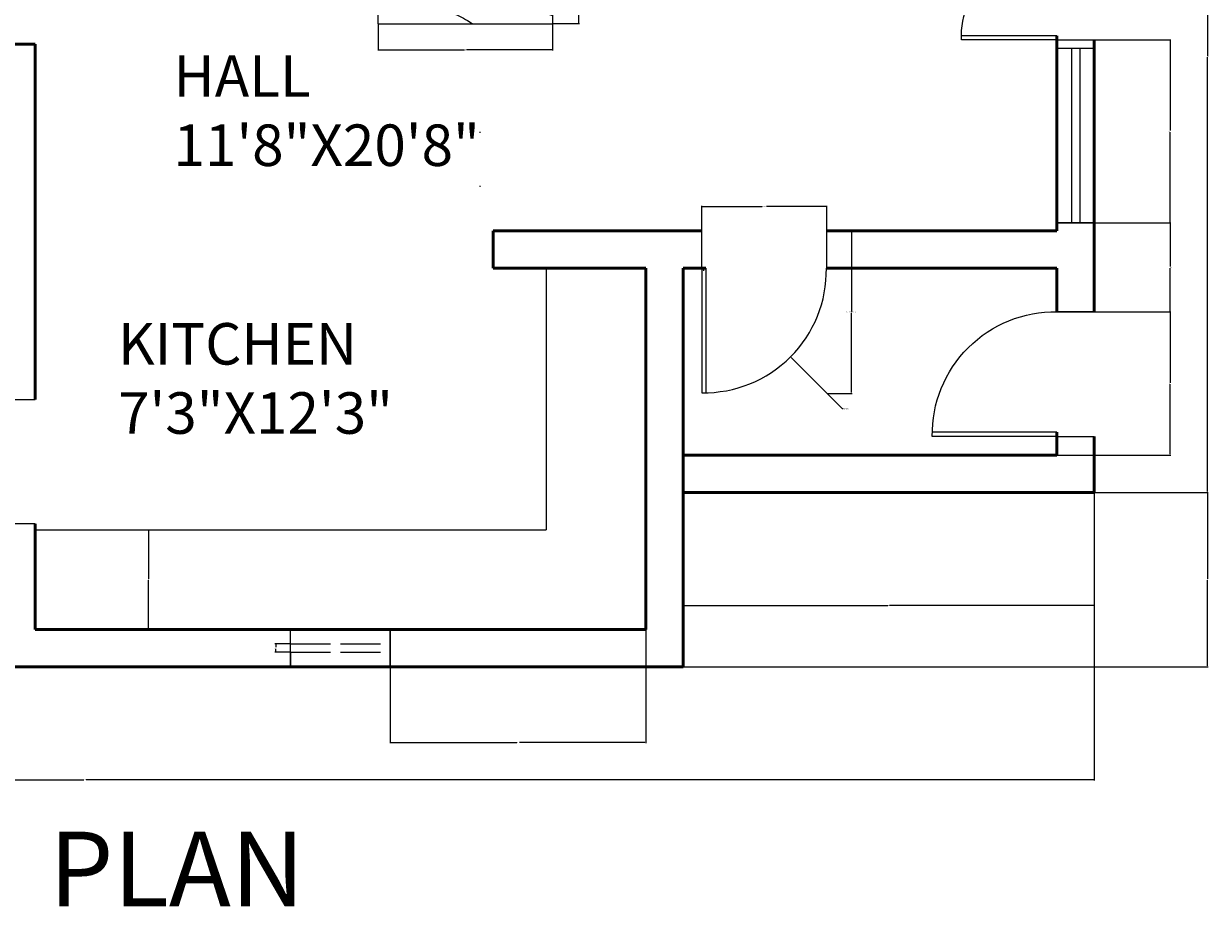
# Model space of a CAD drawing. Units: inches. Extents: x 178 to 719, y 262 to 748.
# Tile 2 of 3: x 434 to 719, y 262 to 475. Entities that reach past the tile are written whole.
import ezdxf

# ---------------------------------------------------------------- set-up
doc = ezdxf.new("R2010")
doc.units = ezdxf.units.IN
doc.linetypes.add('ACAD_ISO02W100', pattern=[15, 12, -3])
for name, color, linetype, lineweight in [('A-ANNO-DIMS', 2, 'Continuous', 18), ('A-ANNO-TEXT', 7, 'Continuous', 35), ('A-AREA-IDEN', 7, 'Continuous', 25), ('A-DOOR', 3, 'Continuous', 25), ('A-FLOR-CASE', 32, 'Continuous', 25), ('A-FURN', 8, 'Continuous', 18), ('A-GLAZ', 4, 'Continuous', 18), ('A-GLAZ-OVHD', 4, 'ACAD_ISO02W100', 18), ('A-WALL', 7, 'Continuous', 50)]:
    doc.layers.add(name, color=color, linetype=linetype, lineweight=lineweight)
doc.styles.get("Standard").update_dxf_attribs({"font": 'arial.ttf'})
doc.dimstyles.get("Standard").update_dxf_attribs({"dimtxt": 0.18, "dimasz": 0.18, "dimexe": 0.18, "dimexo": 0.0625, "dimgap": 0.09, "dimtad": 0, "dimtih": 1, "dimtoh": 1, "dimdec": 4, "dimzin": 0, "dimdsep": 46, "dimtxsty": 'Standard', "dimcen": 0.09, "dimadec": 0, "dimazin": 0, "dimtfac": 1, "dimtdec": 4, "dimtofl": 0, "dimtmove": 0, "dimatfit": 3, "dimfxl": 1, "dimtolj": 1, "dimtzin": 0, "dimarcsym": 0})

# ---------------------------------------------------------------- blocks, each defined once
blk = doc.blocks.new('Table - Square Woodgrain 42 x 42 in.')
blk.add_line((0, -42), (42, -42))
for points in [[(0, -4), (1.704, -4.2172), (3.2358, -4.4188), (4.615, -4.604), (5.8615, -4.7721), (6.9951, -4.9224), (8.0357, -5.0541), (9.0031, -5.1667), (9.9171, -5.2594), (10.7951, -5.3316), (11.6445, -5.3836), (12.4702, -5.4157), (13.277, -5.4283), (14.0698, -5.4217), (14.8535, -5.3964), (15.6331, -5.3526), (16.4133, -5.2908), (17.1986, -5.2103), (17.9913, -5.1062), (18.793, -4.9727), (19.6056, -4.8038), (20.4307, -4.5937), (21.2701, -4.3365), (22.1256, -4.0262), (22.9989, -3.6571), (23.888, -3.2272), (24.7756, -2.7516), (25.6408, -2.2491), (26.4624, -1.7387), (27.2195, -1.2395), (27.891, -0.7703), (28.456, -0.3501), (28.8934, 0.002)], [(0, -42), (0, 0), (42, 0), (42, -42)], [(0, -8), (1.8203, -8.1001), (3.6741, -8.2149), (5.5411, -8.3408), (7.4011, -8.4741), (9.2339, -8.6112), (11.0193, -8.7484), (12.7371, -8.8821), (14.3671, -9.0086), (15.8954, -9.1246), (17.3337, -9.2278), (18.6997, -9.3159), (20.0116, -9.387), (21.2871, -9.4389), (22.5442, -9.4696), (23.8008, -9.477), (25.0749, -9.459), (26.3791, -9.4137), (27.7049, -9.3403), (29.0383, -9.2382), (30.3655, -9.1068), (31.6728, -8.9455), (32.9461, -8.7535), (34.1717, -8.5304), (35.3358, -8.2756), (36.4268, -7.9863), (37.443, -7.6521), (38.3849, -7.2603), (39.253, -6.7986), (40.048, -6.2542), (40.7705, -5.6147), (41.421, -4.8674), (42, -4)], [(42, -12), (39.1784, -12.8621), (36.4519, -13.5654), (33.8246, -14.1294), (31.3004, -14.5731), (28.8832, -14.9161), (26.577, -15.1775), (24.3858, -15.3768), (22.3136, -15.5332), (20.3622, -15.6632), (18.5254, -15.7718), (16.7947, -15.8612), (15.1618, -15.9338), (13.6183, -15.9916), (12.1558, -16.0369), (10.7659, -16.0718), (9.4403, -16.0987), (8.1703, -16.1191), (6.9461, -16.1325), (5.7577, -16.1377), (4.595, -16.1335), (3.4479, -16.1188), (2.3064, -16.0924), (1.1604, -16.0532), (0, -16)], [(42, -16), (37.6529, -16.7365), (33.8802, -17.329), (30.6179, -17.7961), (27.8015, -18.1561), (25.3668, -18.4275), (23.2497, -18.6288), (21.3859, -18.7785), (19.7111, -18.8949), (18.1693, -18.9939), (16.7375, -19.0795), (15.401, -19.1534), (14.1449, -19.217), (12.9544, -19.2717), (11.8148, -19.3191), (10.7113, -19.3606), (9.6291, -19.3976), (8.5534, -19.4323), (7.47, -19.4689), (6.3643, -19.5122), (5.222, -19.5672), (4.0288, -19.6386), (2.7703, -19.7313), (1.4321, -19.8501), (0, -20)], [(0, -24), (3.9243, -23.6805), (7.4766, -23.4138), (10.6891, -23.1954), (13.5943, -23.0205), (16.2247, -22.8847), (18.6125, -22.7832), (20.7903, -22.7116), (22.7903, -22.6651), (24.6563, -22.642), (26.4764, -22.6507), (28.35, -22.7024), (30.3766, -22.8084), (32.6555, -22.98), (35.2861, -23.2283), (38.3678, -23.5645), (42, -24)], [(42, -32), (37.392, -31.017), (33.4585, -30.2231), (30.1291, -29.5949), (27.3334, -29.109), (25.0009, -28.742), (23.0612, -28.4707), (21.4439, -28.2716), (20.0786, -28.1215), (18.8998, -28.0002), (17.8609, -27.9014), (16.9206, -27.8219), (16.0371, -27.7588), (15.1691, -27.709), (14.2748, -27.6693), (13.3128, -27.6368), (12.2415, -27.6083), (11.0295, -27.5824), (9.6867, -27.5643), (8.233, -27.5608), (6.6884, -27.5787), (5.0728, -27.6248), (3.4062, -27.7058), (1.7086, -27.8286), (0, -28)], [(0, -32), (5.4026, -32.5358), (9.9494, -33.019), (13.7424, -33.4553), (16.8834, -33.8505), (19.4743, -34.2106), (21.6171, -34.5413), (23.4136, -34.8486), (24.9657, -35.1382), (26.3614, -35.4156), (27.6332, -35.6841), (28.7995, -35.9467), (29.8788, -36.2064), (30.8897, -36.4661), (31.8507, -36.7288), (32.7802, -36.9973), (33.6968, -37.2747), (34.6175, -37.5635), (35.5531, -37.8651), (36.5128, -38.1805), (37.506, -38.5108), (38.5421, -38.8568), (39.6302, -39.2197), (40.7797, -39.6004), (42, -40)], [(0, -36), (3.0098, -36.2857), (5.5354, -36.5643), (7.6368, -36.8359), (9.374, -37.1009), (10.807, -37.3597), (11.9957, -37.6126), (13.0002, -37.8599), (13.8804, -38.102), (14.6874, -38.3393), (15.4365, -38.5729), (16.1338, -38.8041), (16.7858, -39.0341), (17.3987, -39.264), (17.9787, -39.4952), (18.5322, -39.7288), (19.0655, -39.9662), (19.5832, -40.2081), (20.0842, -40.4544), (20.5657, -40.7046), (21.0249, -40.9581), (21.459, -41.2144), (21.8653, -41.4731), (22.2409, -41.7335), (22.5831, -41.9951)]]:
    blk.add_lwpolyline(points)
blk = doc.blocks.new('DOOR-SWING-30IN')
for p, q in [((0, 0), (-30, 0)), ((0, 0), (9, 0)), ((0, -1), (-30, -1)), ((9, -30), (0, -30))]:
    blk.add_line(p, q)
blk.add_arc((-0.5, -0.5), 29.5, 179.029, 270.971)
blk = doc.blocks.new('WINDOW-42IN')
for p, q in [((0, 0), (-9, 0)), ((-5.5, 0), (-5.5, -42)), ((-3.5, 0), (-3.5, -36)), ((-3.5, 0), (-3.5, -36)), ((-3.5, 0), (-3.5, -42)), ((0, -42), (-9, -42))]:
    blk.add_line(p, q)
blk = doc.blocks.new('WINDOW-24IN-HIGH-GLAZING')
at = {"ltscale": 0.8}
for p, q in [((-2, 0), (-2, -24)), ((0, 0), (0, -24))]:
    blk.add_line(p, q, dxfattribs=at)
blk = doc.blocks.new('DOOR-PAIRED-LEAF-23IN')
for p, q in [((0, 0), (-23, 0)), ((0, 0), (9, 0)), ((0, -1), (-23, -1))]:
    blk.add_line(p, q)
blk.add_arc((-0.5, -0.5), 22.51, 178.727, 271.273)
blk = doc.blocks.new('*D19')
at = {"layer": 'A-ANNO-DIMS', "color": 0, "lineweight": -2, "transparency": 16777216}
for p, q in [((627.4, 424.74), (633.39, 424.74)), ((633.21, 424.56), (633.21, 405.35)), ((633.21, 385.78), (633.21, 404.99)), ((627.4, 385.6), (633.39, 385.6))]:
    blk.add_line(p, q, dxfattribs=at)
at = {"layer": 'A-ANNO-DIMS', "color": 0, "transparency": 16777216}
for points in [[(633.18, 424.56), (633.24, 424.56), (633.21, 424.74)], [(633.18, 385.78), (633.24, 385.78), (633.21, 385.6)]]:
    blk.add_solid(points, dxfattribs=at)
at = {"layer": 'Defpoints', "color": 0, "transparency": 16777216}
for p in [(627.34, 424.74), (633.21, 424.74), (627.34, 385.6)]:
    blk.add_point(p, dxfattribs=at)
at = {"layer": 'A-ANNO-DIMS', "color": 0, "transparency": 16777216, "insert": (633.21, 405.17), "char_height": 0.18, "attachment_point": 5}
blk.add_mtext('\\A1;SWING DOOR 39 TYP.', dxfattribs=at)
blk = doc.blocks.new('*D20')
at = {"layer": 'A-ANNO-DIMS', "color": 0, "lineweight": -2, "transparency": 16777216}
for p, q in [((597.2, 424.8), (597.2, 430.79)), ((627.34, 424.8), (627.34, 430.79)), ((597.38, 430.61), (611.74, 430.61)), ((627.16, 430.61), (612.8, 430.61))]:
    blk.add_line(p, q, dxfattribs=at)
at = {"layer": 'A-ANNO-DIMS', "color": 0, "transparency": 16777216}
for points in [[(597.38, 430.64), (597.38, 430.58), (597.2, 430.61)], [(627.16, 430.64), (627.16, 430.58), (627.34, 430.61)]]:
    blk.add_solid(points, dxfattribs=at)
at = {"layer": 'Defpoints', "color": 0, "transparency": 16777216}
for p in [(597.2, 430.61), (597.2, 424.74), (627.34, 424.74)]:
    blk.add_point(p, dxfattribs=at)
at = {"layer": 'A-ANNO-DIMS', "color": 0, "transparency": 16777216, "insert": (612.27, 430.61), "char_height": 0.18, "attachment_point": 5}
blk.add_mtext('\\A1;30 TYP.', dxfattribs=at)
blk = doc.blocks.new('*D29')
at = {"layer": 'A-ANNO-DIMS', "color": 0, "lineweight": -2, "transparency": 16777216}
for p, q in [((498.2, 323.17), (498.2, 319.46)), ((522.2, 323.17), (522.2, 319.46)), ((498.38, 319.64), (508.74, 319.64)), ((522.02, 319.64), (511.66, 319.64))]:
    blk.add_line(p, q, dxfattribs=at)
at = {"layer": 'A-ANNO-DIMS', "color": 0, "transparency": 16777216}
for points in [[(498.38, 319.67), (498.38, 319.61), (498.2, 319.64)], [(522.02, 319.67), (522.02, 319.61), (522.2, 319.64)]]:
    blk.add_solid(points, dxfattribs=at)
at = {"layer": 'Defpoints', "color": 0, "transparency": 16777216}
for p in [(498.2, 323.24), (522.2, 323.24), (498.2, 319.64)]:
    blk.add_point(p, dxfattribs=at)
at = {"layer": 'A-ANNO-DIMS', "color": 0, "transparency": 16777216, "insert": (510.2, 319.64), "char_height": 0.18, "attachment_point": 5}
blk.add_mtext('\\A1;HIGH WINDOW 24 TYP.', dxfattribs=at)
blk = doc.blocks.new('*D30')
at = {"layer": 'A-ANNO-DIMS', "color": 0, "lineweight": -2, "transparency": 16777216}
for p, q in [((498.14, 325.24), (494.42, 325.24)), ((498.14, 323.24), (494.42, 323.24)), ((494.6, 325.06), (494.6, 324.42)), ((494.6, 323.42), (494.6, 324.06))]:
    blk.add_line(p, q, dxfattribs=at)
at = {"layer": 'A-ANNO-DIMS', "color": 0, "transparency": 16777216}
for points in [[(494.57, 325.06), (494.63, 325.06), (494.6, 325.24)], [(494.57, 323.42), (494.63, 323.42), (494.6, 323.24)]]:
    blk.add_solid(points, dxfattribs=at)
at = {"layer": 'Defpoints', "color": 0, "transparency": 16777216}
for p in [(494.6, 325.24), (498.2, 325.24), (498.2, 323.24)]:
    blk.add_point(p, dxfattribs=at)
at = {"layer": 'A-ANNO-DIMS', "color": 0, "transparency": 16777216, "insert": (494.6, 324.24), "char_height": 0.18, "attachment_point": 5}
blk.add_mtext('\\A1;2 TYP.', dxfattribs=at)
blk = doc.blocks.new('*D39')
at = {"layer": 'A-ANNO-DIMS', "color": 0, "lineweight": -2, "transparency": 16777216}
for p, q in [((561.35, 516.67), (567.77, 516.67)), ((567.59, 516.49), (567.59, 495.85)), ((567.59, 474.85), (567.59, 495.49)), ((561.35, 474.67), (567.77, 474.67))]:
    blk.add_line(p, q, dxfattribs=at)
at = {"layer": 'A-ANNO-DIMS', "color": 0, "transparency": 16777216}
for points in [[(567.56, 516.49), (567.62, 516.49), (567.59, 516.67)], [(567.56, 474.85), (567.62, 474.85), (567.59, 474.67)]]:
    blk.add_solid(points, dxfattribs=at)
at = {"layer": 'Defpoints', "color": 0, "transparency": 16777216}
for p in [(561.29, 516.67), (567.59, 516.67), (561.29, 474.67)]:
    blk.add_point(p, dxfattribs=at)
at = {"layer": 'A-ANNO-DIMS', "color": 0, "transparency": 16777216, "insert": (567.59, 495.67), "char_height": 0.18, "attachment_point": 5}
blk.add_mtext('\\A1;COFFEE TABLE 42', dxfattribs=at)
blk = doc.blocks.new('*D40')
at = {"layer": 'A-ANNO-DIMS', "color": 0, "lineweight": -2, "transparency": 16777216}
for p, q in [((519.29, 474.61), (519.29, 468.19)), ((561.29, 474.61), (561.29, 468.19)), ((519.47, 468.37), (540.07, 468.37)), ((561.11, 468.37), (540.51, 468.37))]:
    blk.add_line(p, q, dxfattribs=at)
at = {"layer": 'A-ANNO-DIMS', "color": 0, "transparency": 16777216}
for points in [[(519.47, 468.4), (519.47, 468.34), (519.29, 468.37)], [(561.11, 468.4), (561.11, 468.34), (561.29, 468.37)]]:
    blk.add_solid(points, dxfattribs=at)
at = {"layer": 'Defpoints', "color": 0, "transparency": 16777216}
for p in [(519.29, 474.67), (561.29, 474.67), (561.29, 468.37)]:
    blk.add_point(p, dxfattribs=at)
at = {"layer": 'A-ANNO-DIMS', "color": 0, "transparency": 16777216, "insert": (540.29, 468.37), "char_height": 0.18, "attachment_point": 5}
blk.add_mtext('\\A1;42', dxfattribs=at)
blk = doc.blocks.new('*D41')
at = {"layer": 'A-ANNO-DIMS', "color": 0, "lineweight": -2, "transparency": 16777216}
for p, q in [((205.7, 385.67), (205.7, 292.31)), ((691.7, 361.67), (691.7, 292.31)), ((205.88, 292.49), (448.41, 292.49)), ((691.52, 292.49), (448.99, 292.49))]:
    blk.add_line(p, q, dxfattribs=at)
at = {"layer": 'A-ANNO-DIMS', "color": 0, "transparency": 16777216}
for points in [[(205.88, 292.52), (205.88, 292.46), (205.7, 292.49)], [(691.52, 292.52), (691.52, 292.46), (691.7, 292.49)]]:
    blk.add_solid(points, dxfattribs=at)
at = {"layer": 'Defpoints', "color": 0, "transparency": 16777216}
for p in [(205.7, 385.74), (691.7, 361.74), (691.7, 292.49)]:
    blk.add_point(p, dxfattribs=at)
at = {"layer": 'A-ANNO-DIMS', "color": 0, "transparency": 16777216, "insert": (448.7, 292.49), "char_height": 0.18, "attachment_point": 5}
blk.add_mtext('\\A1;486', dxfattribs=at)
blk = doc.blocks.new('*D48')
at = {"layer": 'A-ANNO-DIMS', "color": 0, "lineweight": -2, "transparency": 16777216}
for p, q in [((691.76, 361.74), (719.13, 361.74)), ((718.95, 361.56), (718.95, 340.92)), ((718.95, 319.92), (718.95, 340.56)), ((592.76, 319.74), (719.13, 319.74))]:
    blk.add_line(p, q, dxfattribs=at)
at = {"layer": 'A-ANNO-DIMS', "color": 0, "transparency": 16777216}
for points in [[(718.92, 361.56), (718.98, 361.56), (718.95, 361.74)], [(718.92, 319.92), (718.98, 319.92), (718.95, 319.74)]]:
    blk.add_solid(points, dxfattribs=at)
at = {"layer": 'Defpoints', "color": 0, "transparency": 16777216}
for p in [(691.7, 361.74), (718.95, 361.74), (592.7, 319.74)]:
    blk.add_point(p, dxfattribs=at)
at = {"layer": 'A-ANNO-DIMS', "color": 0, "transparency": 16777216, "insert": (718.95, 340.74), "char_height": 0.18, "attachment_point": 5}
blk.add_mtext('\\A1;42', dxfattribs=at)
blk = doc.blocks.new('*D49')
at = {"layer": 'A-ANNO-DIMS', "color": 0, "lineweight": -2, "transparency": 16777216}
for p, q in [((691.76, 571.74), (719.13, 571.74)), ((718.95, 571.56), (718.95, 466.92)), ((718.95, 361.92), (718.95, 466.56)), ((691.76, 361.74), (719.13, 361.74))]:
    blk.add_line(p, q, dxfattribs=at)
at = {"layer": 'A-ANNO-DIMS', "color": 0, "transparency": 16777216}
for points in [[(718.92, 571.56), (718.98, 571.56), (718.95, 571.74)], [(718.92, 361.92), (718.98, 361.92), (718.95, 361.74)]]:
    blk.add_solid(points, dxfattribs=at)
at = {"layer": 'Defpoints', "color": 0, "transparency": 16777216}
for p in [(691.7, 571.74), (691.7, 361.74), (718.95, 361.74)]:
    blk.add_point(p, dxfattribs=at)
at = {"layer": 'A-ANNO-DIMS', "color": 0, "transparency": 16777216, "insert": (718.95, 466.74), "char_height": 0.18, "attachment_point": 5}
blk.add_mtext('\\A1;210', dxfattribs=at)
blk = doc.blocks.new('*D54')
at = {"layer": 'A-ANNO-DIMS', "color": 0, "lineweight": -2, "transparency": 16777216}
for p, q in [((592.7, 361.67), (592.7, 334.31)), ((691.7, 361.67), (691.7, 334.31)), ((592.88, 334.49), (641.98, 334.49)), ((691.52, 334.49), (642.42, 334.49))]:
    blk.add_line(p, q, dxfattribs=at)
at = {"layer": 'A-ANNO-DIMS', "color": 0, "transparency": 16777216}
for points in [[(592.88, 334.52), (592.88, 334.46), (592.7, 334.49)], [(691.52, 334.52), (691.52, 334.46), (691.7, 334.49)]]:
    blk.add_solid(points, dxfattribs=at)
at = {"layer": 'Defpoints', "color": 0, "transparency": 16777216}
for p in [(592.7, 361.74), (691.7, 361.74), (592.7, 334.49)]:
    blk.add_point(p, dxfattribs=at)
at = {"layer": 'A-ANNO-DIMS', "color": 0, "transparency": 16777216, "insert": (642.2, 334.49), "char_height": 0.18, "attachment_point": 5}
blk.add_mtext('\\A1;99', dxfattribs=at)
blk = doc.blocks.new('*D60')
at = {"layer": 'A-ANNO-DIMS', "color": 0, "lineweight": -2, "transparency": 16777216}
for p, q in [((682.76, 405.24), (710.13, 405.24)), ((709.95, 405.06), (709.95, 388.17)), ((709.95, 370.92), (709.95, 387.81)), ((682.76, 370.74), (710.13, 370.74))]:
    blk.add_line(p, q, dxfattribs=at)
at = {"layer": 'A-ANNO-DIMS', "color": 0, "transparency": 16777216}
for points in [[(709.92, 405.06), (709.98, 405.06), (709.95, 405.24)], [(709.92, 370.92), (709.98, 370.92), (709.95, 370.74)]]:
    blk.add_solid(points, dxfattribs=at)
at = {"layer": 'Defpoints', "color": 0, "transparency": 16777216}
for p in [(682.7, 405.24), (682.7, 370.74), (709.95, 370.74)]:
    blk.add_point(p, dxfattribs=at)
at = {"layer": 'A-ANNO-DIMS', "color": 0, "transparency": 16777216, "insert": (709.95, 387.99), "char_height": 0.18, "attachment_point": 5}
blk.add_mtext('\\A1;34.5', dxfattribs=at)
blk = doc.blocks.new('*D61')
at = {"layer": 'A-ANNO-DIMS', "color": 0, "lineweight": -2, "transparency": 16777216}
for p, q in [((682.76, 426.68), (710.13, 426.68)), ((709.95, 426.5), (709.95, 416.14)), ((709.95, 405.42), (709.95, 415.78)), ((682.76, 405.24), (710.13, 405.24))]:
    blk.add_line(p, q, dxfattribs=at)
at = {"layer": 'A-ANNO-DIMS', "color": 0, "transparency": 16777216}
for points in [[(709.92, 426.5), (709.98, 426.5), (709.95, 426.68)], [(709.92, 405.42), (709.98, 405.42), (709.95, 405.24)]]:
    blk.add_solid(points, dxfattribs=at)
at = {"layer": 'Defpoints', "color": 0, "transparency": 16777216}
for p in [(682.7, 426.68), (682.7, 405.24), (709.95, 405.24)]:
    blk.add_point(p, dxfattribs=at)
at = {"layer": 'A-ANNO-DIMS', "color": 0, "transparency": 16777216, "insert": (709.95, 415.96), "char_height": 0.18, "attachment_point": 5}
blk.add_mtext('\\A1;21.44', dxfattribs=at)
blk = doc.blocks.new('*D62')
at = {"layer": 'A-ANNO-DIMS', "color": 0, "lineweight": -2, "transparency": 16777216}
for p, q in [((682.76, 470.74), (710.13, 470.74)), ((709.95, 470.56), (709.95, 448.89)), ((709.95, 426.86), (709.95, 448.53)), ((682.76, 426.68), (710.13, 426.68))]:
    blk.add_line(p, q, dxfattribs=at)
at = {"layer": 'A-ANNO-DIMS', "color": 0, "transparency": 16777216}
for points in [[(709.92, 470.56), (709.98, 470.56), (709.95, 470.74)], [(709.92, 426.86), (709.98, 426.86), (709.95, 426.68)]]:
    blk.add_solid(points, dxfattribs=at)
at = {"layer": 'Defpoints', "color": 0, "transparency": 16777216}
for p in [(682.7, 470.74), (682.7, 426.68), (709.95, 426.68)]:
    blk.add_point(p, dxfattribs=at)
at = {"layer": 'A-ANNO-DIMS', "color": 0, "transparency": 16777216, "insert": (709.95, 448.71), "char_height": 0.18, "attachment_point": 5}
blk.add_mtext('\\A1;44.06', dxfattribs=at)
blk = doc.blocks.new('*D67')
at = {"layer": 'A-ANNO-DIMS', "color": 0, "lineweight": -2, "transparency": 16777216}
for p, q in [((522.2, 328.67), (522.2, 301.31)), ((583.7, 328.67), (583.7, 301.31)), ((522.38, 301.49), (552.63, 301.49)), ((583.52, 301.49), (553.28, 301.49))]:
    blk.add_line(p, q, dxfattribs=at)
at = {"layer": 'A-ANNO-DIMS', "color": 0, "transparency": 16777216}
for points in [[(522.38, 301.52), (522.38, 301.46), (522.2, 301.49)], [(583.52, 301.52), (583.52, 301.46), (583.7, 301.49)]]:
    blk.add_solid(points, dxfattribs=at)
at = {"layer": 'Defpoints', "color": 0, "transparency": 16777216}
for p in [(522.2, 328.74), (583.7, 328.74), (522.2, 301.49)]:
    blk.add_point(p, dxfattribs=at)
at = {"layer": 'A-ANNO-DIMS', "color": 0, "transparency": 16777216, "insert": (552.95, 301.49), "char_height": 0.18, "attachment_point": 5}
blk.add_mtext('\\A1;61.5', dxfattribs=at)
blk = doc.blocks.new('*D68')
at = {"layer": 'A-ANNO-DIMS', "color": 0, "lineweight": -2, "transparency": 16777216}
for p, q in [((436.76, 352.74), (464.13, 352.74)), ((463.95, 352.56), (463.95, 340.92)), ((463.95, 328.92), (463.95, 340.56)), ((436.76, 328.74), (464.13, 328.74))]:
    blk.add_line(p, q, dxfattribs=at)
at = {"layer": 'A-ANNO-DIMS', "color": 0, "transparency": 16777216}
for points in [[(463.92, 352.56), (463.98, 352.56), (463.95, 352.74)], [(463.92, 328.92), (463.98, 328.92), (463.95, 328.74)]]:
    blk.add_solid(points, dxfattribs=at)
at = {"layer": 'Defpoints', "color": 0, "transparency": 16777216}
for p in [(436.7, 352.74), (436.7, 328.74), (463.95, 328.74)]:
    blk.add_point(p, dxfattribs=at)
at = {"layer": 'A-ANNO-DIMS', "color": 0, "transparency": 16777216, "insert": (463.95, 340.74), "char_height": 0.18, "attachment_point": 5}
blk.add_mtext('\\A1;24', dxfattribs=at)
blk = doc.blocks.new('*D71')
at = {"layer": 'A-ANNO-DIMS', "color": 0, "lineweight": -2, "transparency": 16777216}
for p, q in [((597.61, 415.24), (597.79, 415.24)), ((597.7, 415.15), (597.7, 415.33)), ((631.08, 381.86), (618.69, 394.25)), ((631.26, 381.86), (631.08, 381.86))]:
    blk.add_line(p, q, dxfattribs=at)
at = {"layer": 'A-ANNO-DIMS', "color": 0, "transparency": 16777216}
blk.add_solid([(618.71, 394.27), (618.67, 394.23), (618.56, 394.37)], dxfattribs=at)
at = {"layer": 'Defpoints', "color": 0, "transparency": 16777216}
for p in [(597.7, 415.24), (618.56, 394.37)]:
    blk.add_point(p, dxfattribs=at)
at = {"layer": 'A-ANNO-DIMS', "color": 0, "transparency": 16777216, "insert": (632, 381.86), "char_height": 0.18, "attachment_point": 5}
blk.add_mtext('\\A1;6X R29.504', dxfattribs=at)
blk = doc.blocks.new('*D73')
at = {"layer": 'A-ANNO-DIMS', "color": 0, "lineweight": -2, "transparency": 16777216}
for p, q in [((544.03, 629.46), (543.85, 629.46)), ((543.85, 629.46), (543.85, 556.92)), ((543.76, 435.54), (543.94, 435.54)), ((543.85, 435.45), (543.85, 435.63))]:
    blk.add_line(p, q, dxfattribs=at)
at = {"layer": 'A-ANNO-DIMS', "color": 0, "transparency": 16777216}
blk.add_solid([(543.82, 556.92), (543.88, 556.92), (543.85, 556.74)], dxfattribs=at)
at = {"layer": 'Defpoints', "color": 0, "transparency": 16777216}
for p in [(543.85, 556.74), (543.85, 435.54)]:
    blk.add_point(p, dxfattribs=at)
at = {"layer": 'A-ANNO-DIMS', "color": 0, "transparency": 16777216, "insert": (544.51, 629.46), "char_height": 0.18, "attachment_point": 5}
blk.add_mtext('\\A1;R121.2', dxfattribs=at)
blk = doc.blocks.new('*D74')
at = {"layer": 'A-ANNO-DIMS', "color": 0, "lineweight": -2, "transparency": 16777216}
for p, q in [((544.03, 631.29), (543.85, 631.29)), ((543.85, 631.29), (543.85, 562.92)), ((543.76, 448.49), (543.94, 448.49)), ((543.85, 448.4), (543.85, 448.58))]:
    blk.add_line(p, q, dxfattribs=at)
at = {"layer": 'A-ANNO-DIMS', "color": 0, "transparency": 16777216}
blk.add_solid([(543.82, 562.92), (543.88, 562.92), (543.85, 562.74)], dxfattribs=at)
at = {"layer": 'Defpoints', "color": 0, "transparency": 16777216}
for p in [(543.85, 562.74), (543.85, 448.49)]:
    blk.add_point(p, dxfattribs=at)
at = {"layer": 'A-ANNO-DIMS', "color": 0, "transparency": 16777216, "insert": (544.58, 631.29), "char_height": 0.18, "attachment_point": 5}
blk.add_mtext('\\A1;R114.25', dxfattribs=at)

msp = doc.modelspace()

# ---------------------------------------------------------------- linework, layer by layer
at = {"layer": 'A-FLOR-CASE'}
for p in [(559.7008, 415.737), (436.7008, 352.737)]:
    msp.add_line(p, (559.7008, 352.737), dxfattribs=at)
at = {"layer": 'A-GLAZ'}
for p, q in [((498.2008, 319.737), (498.2008, 328.737)), ((522.2008, 319.737), (522.2008, 328.737))]:
    msp.add_line(p, q, dxfattribs=at)
at = {"layer": 'A-WALL'}
for p, q in [((682.7008, 471.737), (682.7008, 424.737)), ((691.7008, 470.737), (691.7008, 415.737)), ((423.2008, 469.737), (436.7008, 469.737)), ((436.7008, 469.737), (436.7008, 415.737)), ((546.9285, 424.737), (597.2008, 424.737)), ((546.9285, 424.737), (546.9285, 415.737)), ((627.2008, 424.737), (682.7008, 424.737)), ((436.7008, 415.737), (436.7008, 385.737)), ((546.9285, 415.737), (583.7008, 415.737)), ((583.7008, 415.737), (583.7008, 328.737)), ((592.7008, 415.737), (592.7008, 319.737)), ((592.7008, 415.737), (598.2008, 415.737)), ((627.2008, 415.737), (682.7008, 415.737)), ((682.7008, 415.737), (682.7008, 405.237)), ((691.7008, 415.737), (691.7008, 405.237)), ((436.7008, 385.737), (436.7008, 384.1411)), ((682.7008, 376.237), (682.7008, 370.737)), ((691.7008, 375.237), (691.7008, 361.737)), ((592.7008, 370.737), (682.7008, 370.737)), ((592.7008, 361.737), (691.7008, 361.737)), ((436.7008, 354.1411), (436.7008, 328.737)), ((436.7008, 328.737), (583.7008, 328.737)), ((343.7008, 319.737), (436.7008, 319.737)), ((436.7008, 319.737), (592.7008, 319.737))]:
    msp.add_line(p, q, dxfattribs=at)

# ---------------------------------------------------------------- block references
at = {"layer": 'A-DOOR', "extrusion": (0, 0, -1), "zscale": -1, "rotation": 180}
for name, p in [('DOOR-PAIRED-LEAF-23IN', (-682.7008, 470.737)), ('DOOR-SWING-30IN', (-682.7008, 375.237))]:
    msp.add_blockref(name, p, dxfattribs=at)
at = {"layer": 'A-DOOR', "rotation": 90.00000000000126}
msp.add_blockref('DOOR-SWING-30IN', (597.2008, 415.737), dxfattribs=at)
at = {"layer": 'A-DOOR'}
msp.add_blockref('DOOR-SWING-30IN', (427.7008, 384.1411), dxfattribs=at)
at = {"layer": 'A-FURN'}
msp.add_blockref('Table - Square Woodgrain 42 x 42 in.', (519.289, 516.6678), dxfattribs=at)
at = {"layer": 'A-GLAZ'}
msp.add_blockref('WINDOW-42IN', (691.7008, 468.6779), dxfattribs=at)
at = {"layer": 'A-GLAZ-OVHD', "rotation": 90}
msp.add_blockref('WINDOW-24IN-HIGH-GLAZING', (498.2008, 325.237), dxfattribs=at)

# ---------------------------------------------------------------- texts
at = {"layer": 'A-ANNO-TEXT', "insert": (440, 280), "char_height": 18, "attachment_point": 1}
msp.add_mtext_dynamic_manual_height_columns('{\\fArial|b1|i0|c0|p34;PLAN}', width=280, gutter_width=12.5, heights=[0], dxfattribs=at)
at = {"layer": 'A-AREA-IDEN', "char_height": 10, "attachment_point": 1}
for s, insert in [('HALL\\P11\'8"X20\'8"', (470, 467.0555)), ('KITCHEN\\P7\'3"X12\'3"', (456.6561, 402.525))]:
    msp.add_mtext_dynamic_manual_height_columns(s, width=98.987328, gutter_width=12.5, heights=[0], dxfattribs=dict(at, insert=insert))

# ---------------------------------------------------------------- dimensions: what is measured, and where the dimension line sits
at = {"layer": 'A-ANNO-DIMS'}
for center, mpoint, override, picture, middle in [((543.8486, 448.487), (543.849, 562.737), {"dimdec": 2, "dimlfac": 1, "dimrnd": 0, "dimzin": 0, "dimdsep": 46, "dimlunit": 2}, '*D74', (544.5797, 631.287)), ((543.8486, 435.5402), (543.849, 556.737), {"dimdec": 1, "dimlfac": 1, "dimrnd": 0, "dimzin": 0, "dimdsep": 46, "dimlunit": 2}, '*D73', (544.5082, 629.4551))]:
    dim = msp.add_radius_dim(center=center, mpoint=mpoint, dimstyle='Standard', override=override, dxfattribs=at)
    dim.commit()
    dim.dimension.update_dxf_attribs({"geometry": picture, "text_midpoint": middle, "dimtype": 164})
for base, p1, p2, angle, override, picture, middle in [((718.9508, 361.737), (691.7008, 571.737), (691.7008, 361.737), 270, {"dimdec": 0, "dimlfac": 1, "dimrnd": 0, "dimzin": 0, "dimdsep": 46, "dimlunit": 2}, '*D49', (718.9508, 466.737)), ((709.9508, 426.6779), (682.7008, 470.737), (682.7008, 426.6779), 270, {"dimdec": 2, "dimlfac": 1, "dimrnd": 0, "dimzin": 0, "dimdsep": 46, "dimlunit": 2}, '*D62', (709.9508, 448.7074)), ((709.9508, 405.237), (682.7008, 426.6779), (682.7008, 405.237), 270, {"dimdec": 2, "dimlfac": 1, "dimrnd": 0, "dimzin": 0, "dimdsep": 46, "dimlunit": 2}, '*D61', (709.9508, 415.9574)), ((709.9508, 370.737), (682.7008, 405.237), (682.7008, 370.737), 270, {"dimdec": 1, "dimlfac": 1, "dimrnd": 0, "dimzin": 0, "dimdsep": 46, "dimlunit": 2}, '*D60', (709.9508, 387.987)), ((718.9508, 361.737), (592.7008, 319.737), (691.7008, 361.737), 90, {"dimdec": 0, "dimlfac": 1, "dimrnd": 0, "dimzin": 0, "dimdsep": 46, "dimlunit": 2}, '*D48', (718.9508, 340.737)), ((592.7008, 334.487), (691.7008, 361.737), (592.7008, 361.737), 180, {"dimdec": 0, "dimlfac": 1, "dimrnd": 0, "dimzin": 0, "dimdsep": 46, "dimlunit": 2}, '*D54', (642.2008, 334.487)), ((463.9508, 328.737), (436.7008, 352.737), (436.7008, 328.737), 270, {"dimdec": 0, "dimlfac": 1, "dimrnd": 0, "dimzin": 0, "dimdsep": 46, "dimlunit": 2}, '*D68', (463.9508, 340.737)), ((522.2008, 301.487), (583.7008, 328.737), (522.2008, 328.737), 180, {"dimdec": 1, "dimlfac": 1, "dimrnd": 0, "dimzin": 0, "dimdsep": 46, "dimlunit": 2}, '*D67', (552.9508, 301.487))]:
    dim = msp.add_linear_dim(base=base, p1=p1, p2=p2, angle=angle, dimstyle='Standard', override=override, dxfattribs=at)
    dim.commit()
    dim.dimension.update_dxf_attribs({"geometry": picture, "text_midpoint": middle})
for base, p1, p2, angle, text, picture, middle in [((567.5893, 516.6698), (561.289, 474.6678), (561.289, 516.6698), 90, 'COFFEE TABLE <>', '*D39', (567.5893, 495.6688)), ((597.2008, 430.6073), (627.3364, 424.737), (597.2008, 424.737), 180, '<> TYP.', '*D20', (612.2686, 430.6073)), ((633.2067, 424.737), (627.3364, 385.6014), (627.3364, 424.737), 90, 'SWING DOOR <> TYP.', '*D19', (633.2067, 405.1692)), ((494.6008, 325.237), (498.2008, 323.237), (498.2008, 325.237), 90, '<> TYP.', '*D30', (494.6008, 324.237)), ((498.2008, 319.637), (522.2008, 323.237), (498.2008, 323.237), 180, 'HIGH WINDOW <> TYP.', '*D29', (510.2008, 319.637))]:
    dim = msp.add_linear_dim(base=base, p1=p1, p2=p2, angle=angle, text=text, dimstyle='Standard', override={"dimdec": 0, "dimlfac": 1, "dimrnd": 0, "dimzin": 0, "dimdsep": 46, "dimlunit": 2}, dxfattribs=at)
    dim.commit()
    dim.dimension.update_dxf_attribs({"geometry": picture, "text_midpoint": middle})
for base, p1, p2, picture, middle in [((561.289, 468.3675), (519.289, 474.6678), (561.289, 474.6678), '*D40', (540.289, 468.3675)), ((691.7008, 292.487), (205.7008, 385.737), (691.7008, 361.737), '*D41', (448.7008, 292.487))]:
    dim = msp.add_linear_dim(base=base, p1=p1, p2=p2, dimstyle='Standard', override={"dimdec": 0, "dimlfac": 1, "dimrnd": 0, "dimzin": 0, "dimdsep": 46, "dimlunit": 2}, dxfattribs=at)
    dim.commit()
    dim.dimension.update_dxf_attribs({"geometry": picture, "text_midpoint": middle})
dim = msp.add_radius_dim(center=(597.7008, 415.237), mpoint=(618.5631, 394.3739), text='6X <>', dimstyle='Standard', override={"dimdec": 3, "dimlfac": 1, "dimrnd": 0, "dimzin": 0, "dimdsep": 46, "dimlunit": 2}, dxfattribs=at)
dim.commit()
dim.dimension.update_dxf_attribs({"geometry": '*D71', "text_midpoint": (632.0037, 381.8561), "dimtype": 164})

doc.saveas('drawing.dxf')
